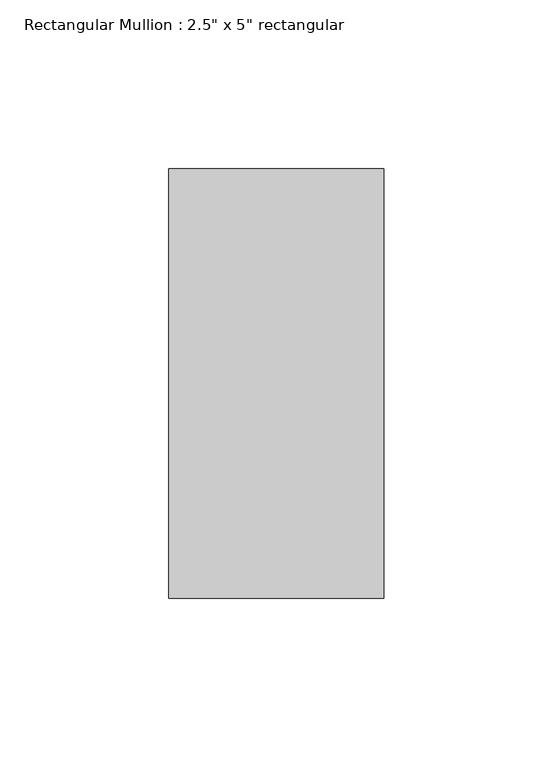
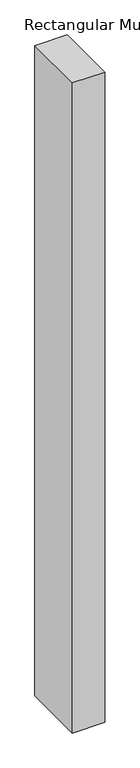
"""IFC4 building model written with IfcOpenShell, lengths in millimetres: member geometry."""

from ifc_helpers import new_model, si_unit, frame, origin, place, context, project, spatial, polyline, outline, extrude, source, transform, mapped, element, save


def member_b07cc7a9(model_context):
    return source(origin(), model_context, "Body", "SweptSolid", [
        extrude(outline(polyline([(0.0, 63.5), (0.0, -63.5), (-63.5, -63.5), (-63.5, 63.5), (0.0, 63.5)])), frame((0.0, 0.0, -1343.8279521), z_axis=(0.0, 0.0, 1.0), x_axis=(1.0, 0.0, 0.0)), (0.0, 0.0, 1.0), 1343.8279521),
    ])


if __name__ == "__main__":
    model = new_model("IFC4")
    model_context = context("Model", 3, world=origin())
    ifc_project = project(units=[si_unit("LENGTHUNIT", "METRE", prefix="MILLI")], contexts=[model_context])
    site = spatial("IfcSite", under=ifc_project)
    building = spatial("IfcBuilding", under=site)
    placement = place(None, origin())
    member_shape = member_b07cc7a9(model_context)
    element("IfcMember", 1, ObjectType="Rectangular Mullion : 2.5\" x 5\" rectangular", at=placement, inside=building, context=model_context, shape_type="MappedRepresentation", body=[
        mapped(member_shape, transform((0.0, 0.0, 0.0), x_axis=(1.0, 0.0, 0.0), y_axis=(0.0, 1.0, 0.0), z_axis=(0.0, 0.0, 1.0))),
    ])
    save(model, "model.ifc")

# Revit data of these elements
# Type "Rectangular Mullion : 2.5\" x 5\" rectangular"
#   built-in parameter 1007304 = 0.416667 (stored number, unit not read)
#   built-in parameter 1007301 = 0.104167 (stored number, unit not read)
#   built-in parameter 1007300 = 0.104167 (stored number, unit not read)
# Element 1 (IfcMember, "Rectangular Mullion : 2.5\" x 5\" rectangular")
#   Materials on its faces: "Aluminum"
# Materials
#   "Aluminum": class "Metal", colour RGB 247 247 247, transparency 0, Description = "Aluminum 6061", Cost = 0
